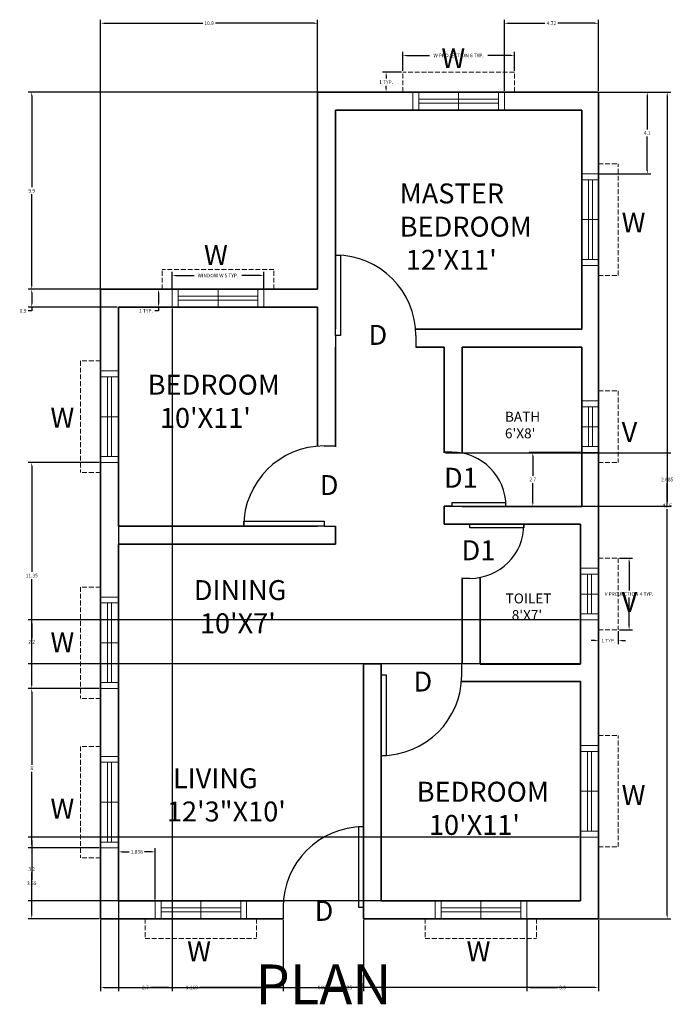
# Model space of a CAD drawing. Units: inches. Extents: x -193.8 to -127.9, y -122.4 to -72.3.
# Tile 1 of 2: x -193.8 to -161, y -122.4 to -73. Entities that reach past the tile are written whole.
import ezdxf

# ---------------------------------------------------------------- set-up
doc = ezdxf.new("R2010")
doc.units = ezdxf.units.IN
doc.header["$LTSCALE"] = 0.2
doc.header["$MEASUREMENT"] = 0
doc.linetypes.add('ACAD_ISO02W100', pattern=[15, 12, -3])
for name, color, linetype, lineweight in [('A-ANNO-DIMS', 2, 'Continuous', 18), ('A-ANNO-TEXT', 7, 'Continuous', 18), ('A-ANNO-TITL', 1, 'Continuous', 35), ('A-AREA-IDEN', 7, 'Continuous', 18), ('A-DOOR', 4, 'Continuous', 25), ('A-GLAZ', 4, 'Continuous', 18), ('A-GLAZ-OVHD', 8, 'ACAD_ISO02W100', 13), ('A-WALL', 7, 'Continuous', 35)]:
    doc.layers.add(name, color=color, linetype=linetype, lineweight=lineweight)
doc.styles.get("Standard").update_dxf_attribs({"font": 'arial.ttf'})
doc.dimstyles.get("Standard").update_dxf_attribs({"dimtxt": 0.18, "dimasz": 0.18, "dimexe": 0.18, "dimexo": 0.0625, "dimgap": 0.09, "dimtad": 0, "dimtih": 1, "dimtoh": 1, "dimdec": 1, "dimzin": 0, "dimdsep": 46, "dimlunit": 4, "dimtxsty": 'Standard', "dimcen": 0.09, "dimadec": 0, "dimazin": 0, "dimtfac": 1, "dimtdec": 1, "dimtofl": 0, "dimtmove": 0, "dimatfit": 3, "dimfxl": 1, "dimtolj": 1, "dimtzin": 0, "dimarcsym": 0})

# ---------------------------------------------------------------- blocks, each defined once
blk = doc.blocks.new('*U2')
for p, q in [((-700, 0), (-700, -100)), ((0, 0), (0, -100))]:
    blk.add_line(p, q)
blk.add_lwpolyline([(0, 0), (0, 700), (-43.75, 700), (-43.75, 0)], close=True)
blk.add_arc((0, 0), 700, 90, 180)
blk = doc.blocks.new('*U5')
for p, q in [((0, 0), (0, -100)), ((700, 0), (700, -100))]:
    blk.add_line(p, q)
blk.add_lwpolyline([(0, 0), (0, 700), (43.75, 700), (43.75, 0)], close=True)
blk.add_arc((0, 0), 700, 0, 90)
blk = doc.blocks.new('*U6')
for p, q in [((-700, 0), (-700, -100)), ((0, 0), (0, -100))]:
    blk.add_line(p, q)
blk.add_lwpolyline([(0, 0), (0, 700), (-43.75, 700), (-43.75, 0)], close=True)
blk.add_arc((0, 0), 700, 90, 180)
blk = doc.blocks.new('WIN-W-PLAN')
for p, q in [((0, 0.9), (0, 0)), ((0.3, 0.9), (0.3, 0)), ((0.3, 0.55), (4.3, 0.55)), ((2.3, 0.9), (2.3, 0)), ((4.3, 0.9), (4.3, 0)), ((4.6, 0.9), (4.6, 0)), ((0.3, 0.35), (4.3, 0.35))]:
    blk.add_line(p, q)
blk = doc.blocks.new('WIN-W-PROJECTION')
at = {"ltscale": 0.1}
for p, q in [((0.5, 1), (0, 1)), ((0, 1), (0, 0)), ((5.1, 1), (5.6, 1)), ((5.6, 1), (5.6, 0)), ((0, 0), (5.6, 0))]:
    blk.add_line(p, q, dxfattribs=at)
blk = doc.blocks.new('VENT-V-PROJECTION')
at = {"ltscale": 0.1}
for p, q in [((0, 3.1), (0, 3.6)), ((0, 3.6), (1, 3.6)), ((1, 3.6), (1, 0)), ((0, 0.5), (0, 0)), ((0, 0), (1, 0))]:
    blk.add_line(p, q, dxfattribs=at)
blk = doc.blocks.new('*D13')
at = {"layer": 'A-ANNO-DIMS', "color": 0, "lineweight": -2, "ltscale": 0.2, "transparency": 16777216}
for p, q in [((-186.171, -86.486), (-186.171, -85.678)), ((-185.991, -85.858), (-185.073, -85.858)), ((-181.751, -85.858), (-182.669, -85.858)), ((-181.571, -86.486), (-181.571, -85.678))]:
    blk.add_line(p, q, dxfattribs=at)
at = {"layer": 'A-ANNO-DIMS', "color": 0, "ltscale": 0.2, "transparency": 16777216}
for points in [[(-185.991, -85.828), (-185.991, -85.888), (-186.171, -85.858)], [(-181.751, -85.828), (-181.751, -85.888), (-181.571, -85.858)]]:
    blk.add_solid(points, dxfattribs=at)
at = {"layer": 'Defpoints', "color": 0, "ltscale": 0.2, "transparency": 16777216}
for p in [(-186.171, -85.858), (-186.171, -86.548), (-181.571, -86.548)]:
    blk.add_point(p, dxfattribs=at)
at = {"layer": 'A-ANNO-DIMS', "color": 0, "ltscale": 0.2, "transparency": 16777216, "insert": (-183.871, -85.858), "char_height": 0.18, "attachment_point": 5}
blk.add_mtext('\\A1;WINDOW W 5 TYP.', dxfattribs=at)
blk = doc.blocks.new('*D14')
at = {"layer": 'A-ANNO-DIMS', "color": 0, "lineweight": -2, "ltscale": 0.2, "transparency": 16777216}
for p, q in [((-186.234, -86.548), (-187.041, -86.548)), ((-186.861, -86.728), (-186.861, -87.268)), ((-186.234, -87.448), (-187.041, -87.448)), ((-186.861, -87.448), (-186.861, -87.628)), ((-186.861, -87.628), (-187.041, -87.628))]:
    blk.add_line(p, q, dxfattribs=at)
at = {"layer": 'A-ANNO-DIMS', "color": 0, "ltscale": 0.2, "transparency": 16777216}
for points in [[(-186.891, -86.728), (-186.831, -86.728), (-186.861, -86.548)], [(-186.891, -87.268), (-186.831, -87.268), (-186.861, -87.448)]]:
    blk.add_solid(points, dxfattribs=at)
at = {"layer": 'Defpoints', "color": 0, "ltscale": 0.2, "transparency": 16777216}
for p in [(-186.171, -86.548), (-186.861, -87.448), (-186.171, -87.448)]:
    blk.add_point(p, dxfattribs=at)
at = {"layer": 'A-ANNO-DIMS', "color": 0, "ltscale": 0.2, "transparency": 16777216, "insert": (-187.491, -87.628), "char_height": 0.18, "attachment_point": 5}
blk.add_mtext('\\A1;1 TYP.', dxfattribs=at)
blk = doc.blocks.new('*D15')
at = {"layer": 'A-ANNO-DIMS', "color": 0, "lineweight": -2, "ltscale": 0.2, "transparency": 16777216}
for p, q in [((-174.591, -75.586), (-174.591, -74.628)), ((-168.991, -75.586), (-168.991, -74.628)), ((-174.411, -74.808), (-173.252, -74.808)), ((-169.171, -74.808), (-170.331, -74.808))]:
    blk.add_line(p, q, dxfattribs=at)
at = {"layer": 'A-ANNO-DIMS', "color": 0, "ltscale": 0.2, "transparency": 16777216}
for points in [[(-174.411, -74.778), (-174.411, -74.838), (-174.591, -74.808)], [(-169.171, -74.778), (-169.171, -74.838), (-168.991, -74.808)]]:
    blk.add_solid(points, dxfattribs=at)
at = {"layer": 'Defpoints', "color": 0, "ltscale": 0.2, "transparency": 16777216}
for p in [(-174.591, -74.808), (-174.591, -75.648), (-168.991, -75.648)]:
    blk.add_point(p, dxfattribs=at)
at = {"layer": 'A-ANNO-DIMS', "color": 0, "ltscale": 0.2, "transparency": 16777216, "insert": (-171.791, -74.808), "char_height": 0.18, "attachment_point": 5}
blk.add_mtext('\\A1;W PROJECTION 6 TYP.', dxfattribs=at)
blk = doc.blocks.new('*D16')
at = {"layer": 'A-ANNO-DIMS', "color": 0, "lineweight": -2, "ltscale": 0.2, "transparency": 16777216}
for p, q in [((-174.654, -75.648), (-175.611, -75.648)), ((-175.431, -75.828), (-175.431, -75.968)), ((-175.431, -76.468), (-175.431, -76.329)), ((-174.654, -76.648), (-175.611, -76.648))]:
    blk.add_line(p, q, dxfattribs=at)
at = {"layer": 'A-ANNO-DIMS', "color": 0, "ltscale": 0.2, "transparency": 16777216}
for points in [[(-175.461, -75.828), (-175.401, -75.828), (-175.431, -75.648)], [(-175.461, -76.468), (-175.401, -76.468), (-175.431, -76.648)]]:
    blk.add_solid(points, dxfattribs=at)
at = {"layer": 'Defpoints', "color": 0, "ltscale": 0.2, "transparency": 16777216}
for p in [(-174.591, -75.648), (-175.431, -76.648), (-174.591, -76.648)]:
    blk.add_point(p, dxfattribs=at)
at = {"layer": 'A-ANNO-DIMS', "color": 0, "ltscale": 0.2, "transparency": 16777216, "insert": (-175.431, -76.148), "char_height": 0.18, "attachment_point": 5}
blk.add_mtext('\\A1;1 TYP.', dxfattribs=at)
blk = doc.blocks.new('*D17')
at = {"layer": 'A-ANNO-DIMS', "color": 0, "lineweight": -2, "ltscale": 0.2, "transparency": 16777216}
for p, q in [((-163.709, -100.048), (-163.051, -100.048)), ((-163.231, -100.228), (-163.231, -101.665)), ((-163.231, -103.468), (-163.231, -102.031)), ((-163.709, -103.648), (-163.051, -103.648))]:
    blk.add_line(p, q, dxfattribs=at)
at = {"layer": 'A-ANNO-DIMS', "color": 0, "ltscale": 0.2, "transparency": 16777216}
for points in [[(-163.261, -100.228), (-163.201, -100.228), (-163.231, -100.048)], [(-163.261, -103.468), (-163.201, -103.468), (-163.231, -103.648)]]:
    blk.add_solid(points, dxfattribs=at)
at = {"layer": 'Defpoints', "color": 0, "ltscale": 0.2, "transparency": 16777216}
for p in [(-163.771, -100.048), (-163.231, -100.048), (-163.771, -103.648)]:
    blk.add_point(p, dxfattribs=at)
at = {"layer": 'A-ANNO-DIMS', "color": 0, "ltscale": 0.2, "transparency": 16777216, "insert": (-163.231, -101.848), "char_height": 0.18, "attachment_point": 5}
blk.add_mtext('\\A1;V PROJECTION 4 TYP.', dxfattribs=at)
blk = doc.blocks.new('*D18')
at = {"layer": 'A-ANNO-DIMS', "color": 0, "lineweight": -2, "ltscale": 0.2, "transparency": 16777216}
for p, q in [((-164.771, -103.711), (-164.771, -104.368)), ((-163.771, -103.711), (-163.771, -104.368)), ((-164.951, -104.188), (-165.131, -104.188)), ((-163.591, -104.188), (-163.411, -104.188))]:
    blk.add_line(p, q, dxfattribs=at)
at = {"layer": 'A-ANNO-DIMS', "color": 0, "ltscale": 0.2, "transparency": 16777216}
for points in [[(-164.951, -104.158), (-164.951, -104.218), (-164.771, -104.188)], [(-163.591, -104.158), (-163.591, -104.218), (-163.771, -104.188)]]:
    blk.add_solid(points, dxfattribs=at)
at = {"layer": 'Defpoints', "color": 0, "ltscale": 0.2, "transparency": 16777216}
for p in [(-164.771, -103.648), (-163.771, -103.648), (-163.771, -104.188)]:
    blk.add_point(p, dxfattribs=at)
at = {"layer": 'A-ANNO-DIMS', "color": 0, "ltscale": 0.2, "transparency": 16777216, "insert": (-164.271, -104.188), "char_height": 0.18, "attachment_point": 5}
blk.add_mtext('\\A1;1 TYP.', dxfattribs=at)
blk = doc.blocks.new('*D25')
at = {"layer": 'A-ANNO-DIMS', "color": 0, "lineweight": -2, "ltscale": 0.2, "transparency": 16777216}
for p, q in [((-189.771, -118.211), (-189.771, -121.783)), ((-164.771, -118.211), (-164.771, -121.783)), ((-189.591, -121.603), (-177.492, -121.603)), ((-164.951, -121.603), (-177.05, -121.603))]:
    blk.add_line(p, q, dxfattribs=at)
at = {"layer": 'A-ANNO-DIMS', "color": 0, "ltscale": 0.2, "transparency": 16777216}
for points in [[(-189.591, -121.573), (-189.591, -121.633), (-189.771, -121.603)], [(-164.951, -121.573), (-164.951, -121.633), (-164.771, -121.603)]]:
    blk.add_solid(points, dxfattribs=at)
at = {"layer": 'Defpoints', "color": 0, "ltscale": 0.2, "transparency": 16777216}
for p in [(-189.771, -118.148), (-164.771, -118.148), (-164.771, -121.603)]:
    blk.add_point(p, dxfattribs=at)
at = {"layer": 'A-ANNO-DIMS', "color": 0, "ltscale": 0.2, "transparency": 16777216, "insert": (-177.271, -121.603), "char_height": 0.18, "attachment_point": 5}
blk.add_mtext('\\A1;25', dxfattribs=at)
blk = doc.blocks.new('*D26')
at = {"layer": 'A-ANNO-DIMS', "color": 0, "lineweight": -2, "ltscale": 0.2, "transparency": 16777216}
for p, q in [((-164.709, -76.648), (-161.136, -76.648)), ((-161.316, -76.828), (-161.316, -97.216)), ((-161.316, -117.968), (-161.316, -97.58)), ((-164.709, -118.148), (-161.136, -118.148))]:
    blk.add_line(p, q, dxfattribs=at)
at = {"layer": 'A-ANNO-DIMS', "color": 0, "ltscale": 0.2, "transparency": 16777216}
for points in [[(-161.346, -76.828), (-161.286, -76.828), (-161.316, -76.648)], [(-161.346, -117.968), (-161.286, -117.968), (-161.316, -118.148)]]:
    blk.add_solid(points, dxfattribs=at)
at = {"layer": 'Defpoints', "color": 0, "ltscale": 0.2, "transparency": 16777216}
for p in [(-164.771, -76.648), (-161.316, -76.648), (-164.771, -118.148)]:
    blk.add_point(p, dxfattribs=at)
at = {"layer": 'A-ANNO-DIMS', "color": 0, "ltscale": 0.2, "transparency": 16777216, "insert": (-161.316, -97.398), "char_height": 0.18, "attachment_point": 5}
blk.add_mtext('\\A1;41.5', dxfattribs=at)
blk = doc.blocks.new('*D27')
at = {"layer": 'A-ANNO-DIMS', "color": 0, "lineweight": -2, "ltscale": 0.2, "transparency": 16777216}
for p, q in [((-189.771, -86.486), (-189.771, -73.013)), ((-178.871, -86.486), (-178.871, -73.013)), ((-189.591, -73.193), (-184.637, -73.193)), ((-179.051, -73.193), (-184.006, -73.193))]:
    blk.add_line(p, q, dxfattribs=at)
at = {"layer": 'A-ANNO-DIMS', "color": 0, "ltscale": 0.2, "transparency": 16777216}
for points in [[(-189.591, -73.163), (-189.591, -73.223), (-189.771, -73.193)], [(-179.051, -73.163), (-179.051, -73.223), (-178.871, -73.193)]]:
    blk.add_solid(points, dxfattribs=at)
at = {"layer": 'Defpoints', "color": 0, "ltscale": 0.2, "transparency": 16777216}
for p in [(-178.871, -73.193), (-189.771, -86.548), (-178.871, -86.548)]:
    blk.add_point(p, dxfattribs=at)
at = {"layer": 'A-ANNO-DIMS', "color": 0, "ltscale": 0.2, "transparency": 16777216, "insert": (-184.321, -73.193), "char_height": 0.18, "attachment_point": 5}
blk.add_mtext('\\A1;10.9', dxfattribs=at)
blk = doc.blocks.new('*D28')
at = {"layer": 'A-ANNO-DIMS', "color": 0, "lineweight": -2, "ltscale": 0.2, "transparency": 16777216}
for p, q in [((-178.934, -76.648), (-193.406, -76.648)), ((-193.226, -76.828), (-193.226, -81.416)), ((-193.226, -86.368), (-193.226, -81.78)), ((-178.934, -86.548), (-193.406, -86.548))]:
    blk.add_line(p, q, dxfattribs=at)
at = {"layer": 'A-ANNO-DIMS', "color": 0, "ltscale": 0.2, "transparency": 16777216}
for points in [[(-193.256, -76.828), (-193.196, -76.828), (-193.226, -76.648)], [(-193.256, -86.368), (-193.196, -86.368), (-193.226, -86.548)]]:
    blk.add_solid(points, dxfattribs=at)
at = {"layer": 'Defpoints', "color": 0, "ltscale": 0.2, "transparency": 16777216}
for p in [(-193.226, -76.648), (-178.871, -76.648), (-178.871, -86.548)]:
    blk.add_point(p, dxfattribs=at)
at = {"layer": 'A-ANNO-DIMS', "color": 0, "ltscale": 0.2, "transparency": 16777216, "insert": (-193.226, -81.598), "char_height": 0.18, "attachment_point": 5}
blk.add_mtext('\\A1;9.9', dxfattribs=at)
blk = doc.blocks.new('*D29')
at = {"layer": 'A-ANNO-DIMS', "color": 0, "lineweight": -2, "ltscale": 0.2, "transparency": 16777216}
for p, q in [((-189.771, -118.211), (-189.771, -121.783)), ((-180.602, -118.211), (-180.602, -121.783)), ((-189.591, -121.603), (-185.581, -121.603)), ((-180.782, -121.603), (-184.793, -121.603))]:
    blk.add_line(p, q, dxfattribs=at)
at = {"layer": 'A-ANNO-DIMS', "color": 0, "ltscale": 0.2, "transparency": 16777216}
for points in [[(-189.591, -121.573), (-189.591, -121.633), (-189.771, -121.603)], [(-180.782, -121.573), (-180.782, -121.633), (-180.602, -121.603)]]:
    blk.add_solid(points, dxfattribs=at)
at = {"layer": 'Defpoints', "color": 0, "ltscale": 0.2, "transparency": 16777216}
for p in [(-189.771, -118.148), (-180.602, -118.148), (-180.602, -121.603)]:
    blk.add_point(p, dxfattribs=at)
at = {"layer": 'A-ANNO-DIMS', "color": 0, "ltscale": 0.2, "transparency": 16777216, "insert": (-185.187, -121.603), "char_height": 0.18, "attachment_point": 5}
blk.add_mtext('\\A1;9.169', dxfattribs=at)
blk = doc.blocks.new('*D30')
at = {"layer": 'A-ANNO-DIMS', "color": 0, "lineweight": -2, "ltscale": 0.2, "transparency": 16777216}
for p, q in [((-180.602, -118.211), (-180.602, -121.783)), ((-176.571, -118.211), (-176.571, -121.783)), ((-180.422, -121.603), (-178.967, -121.603)), ((-176.751, -121.603), (-178.207, -121.603))]:
    blk.add_line(p, q, dxfattribs=at)
at = {"layer": 'A-ANNO-DIMS', "color": 0, "ltscale": 0.2, "transparency": 16777216}
for points in [[(-180.422, -121.573), (-180.422, -121.633), (-180.602, -121.603)], [(-176.751, -121.573), (-176.751, -121.633), (-176.571, -121.603)]]:
    blk.add_solid(points, dxfattribs=at)
at = {"layer": 'Defpoints', "color": 0, "ltscale": 0.2, "transparency": 16777216}
for p in [(-180.602, -118.148), (-176.571, -118.148), (-176.571, -121.603)]:
    blk.add_point(p, dxfattribs=at)
at = {"layer": 'A-ANNO-DIMS', "color": 0, "ltscale": 0.2, "transparency": 16777216, "insert": (-178.587, -121.603), "char_height": 0.18, "attachment_point": 5}
blk.add_mtext('\\A1;4.031', dxfattribs=at)
blk = doc.blocks.new('*D31')
at = {"layer": 'A-ANNO-DIMS', "color": 0, "lineweight": -2, "ltscale": 0.2, "transparency": 16777216}
for p, q in [((-172.449, -94.756), (-161.136, -94.756)), ((-161.316, -94.936), (-161.316, -95.917)), ((-161.316, -97.261), (-161.316, -96.281)), ((-172.449, -97.441), (-161.136, -97.441))]:
    blk.add_line(p, q, dxfattribs=at)
at = {"layer": 'A-ANNO-DIMS', "color": 0, "ltscale": 0.2, "transparency": 16777216}
for points in [[(-161.346, -94.936), (-161.286, -94.936), (-161.316, -94.756)], [(-161.346, -97.261), (-161.286, -97.261), (-161.316, -97.441)]]:
    blk.add_solid(points, dxfattribs=at)
at = {"layer": 'Defpoints', "color": 0, "ltscale": 0.2, "transparency": 16777216}
for p in [(-172.511, -94.756), (-172.511, -97.441), (-161.316, -97.441)]:
    blk.add_point(p, dxfattribs=at)
at = {"layer": 'A-ANNO-DIMS', "color": 0, "ltscale": 0.2, "transparency": 16777216, "insert": (-161.316, -96.099), "char_height": 0.18, "attachment_point": 5}
blk.add_mtext('\\A1;2.685', dxfattribs=at)
blk = doc.blocks.new('*D32')
at = {"layer": 'A-ANNO-DIMS', "color": 0, "lineweight": -2, "ltscale": 0.2, "transparency": 16777216}
for p, q in [((-189.834, -86.548), (-193.406, -86.548)), ((-193.226, -86.728), (-193.226, -87.268)), ((-188.934, -87.448), (-193.406, -87.448)), ((-193.226, -87.448), (-193.226, -87.628)), ((-193.226, -87.628), (-193.406, -87.628))]:
    blk.add_line(p, q, dxfattribs=at)
at = {"layer": 'A-ANNO-DIMS', "color": 0, "ltscale": 0.2, "transparency": 16777216}
for points in [[(-193.256, -86.728), (-193.196, -86.728), (-193.226, -86.548)], [(-193.256, -87.268), (-193.196, -87.268), (-193.226, -87.448)]]:
    blk.add_solid(points, dxfattribs=at)
at = {"layer": 'Defpoints', "color": 0, "ltscale": 0.2, "transparency": 16777216}
for p in [(-189.771, -86.548), (-193.226, -87.448), (-188.871, -87.448)]:
    blk.add_point(p, dxfattribs=at)
at = {"layer": 'A-ANNO-DIMS', "color": 0, "ltscale": 0.2, "transparency": 16777216, "insert": (-193.66, -87.628), "char_height": 0.18, "attachment_point": 5}
blk.add_mtext('\\A1;0.9', dxfattribs=at)
blk = doc.blocks.new('*D33')
at = {"layer": 'A-ANNO-DIMS', "color": 0, "lineweight": -2, "ltscale": 0.2, "transparency": 16777216}
for p, q in [((-189.834, -114.598), (-193.406, -114.598)), ((-193.226, -114.778), (-193.226, -116.191)), ((-193.226, -117.968), (-193.226, -116.555)), ((-189.834, -118.148), (-193.406, -118.148))]:
    blk.add_line(p, q, dxfattribs=at)
at = {"layer": 'A-ANNO-DIMS', "color": 0, "ltscale": 0.2, "transparency": 16777216}
for points in [[(-193.256, -114.778), (-193.196, -114.778), (-193.226, -114.598)], [(-193.256, -117.968), (-193.196, -117.968), (-193.226, -118.148)]]:
    blk.add_solid(points, dxfattribs=at)
at = {"layer": 'Defpoints', "color": 0, "ltscale": 0.2, "transparency": 16777216}
for p in [(-193.226, -114.598), (-189.771, -114.598), (-189.771, -118.148)]:
    blk.add_point(p, dxfattribs=at)
at = {"layer": 'A-ANNO-DIMS', "color": 0, "ltscale": 0.2, "transparency": 16777216, "insert": (-193.226, -116.373), "char_height": 0.18, "attachment_point": 5}
blk.add_mtext('\\A1;3.55', dxfattribs=at)
blk = doc.blocks.new('*D34')
at = {"layer": 'A-ANNO-DIMS', "color": 0, "lineweight": -2, "ltscale": 0.2, "transparency": 16777216}
for p, q in [((-189.834, -106.598), (-193.406, -106.598)), ((-193.226, -106.778), (-193.226, -110.416)), ((-193.226, -114.418), (-193.226, -110.78)), ((-189.834, -114.598), (-193.406, -114.598))]:
    blk.add_line(p, q, dxfattribs=at)
at = {"layer": 'A-ANNO-DIMS', "color": 0, "ltscale": 0.2, "transparency": 16777216}
for points in [[(-193.256, -106.778), (-193.196, -106.778), (-193.226, -106.598)], [(-193.256, -114.418), (-193.196, -114.418), (-193.226, -114.598)]]:
    blk.add_solid(points, dxfattribs=at)
at = {"layer": 'Defpoints', "color": 0, "ltscale": 0.2, "transparency": 16777216}
for p in [(-193.226, -106.598), (-189.771, -106.598), (-189.771, -114.598)]:
    blk.add_point(p, dxfattribs=at)
at = {"layer": 'A-ANNO-DIMS', "color": 0, "ltscale": 0.2, "transparency": 16777216, "insert": (-193.226, -110.598), "char_height": 0.18, "attachment_point": 5}
blk.add_mtext('\\A1;8', dxfattribs=at)
blk = doc.blocks.new('*D35')
at = {"layer": 'A-ANNO-DIMS', "color": 0, "lineweight": -2, "ltscale": 0.2, "transparency": 16777216}
for p, q in [((-189.834, -95.248), (-193.406, -95.248)), ((-193.226, -95.428), (-193.226, -100.741)), ((-193.226, -106.418), (-193.226, -101.105)), ((-189.834, -106.598), (-193.406, -106.598))]:
    blk.add_line(p, q, dxfattribs=at)
at = {"layer": 'A-ANNO-DIMS', "color": 0, "ltscale": 0.2, "transparency": 16777216}
for points in [[(-193.256, -95.428), (-193.196, -95.428), (-193.226, -95.248)], [(-193.256, -106.418), (-193.196, -106.418), (-193.226, -106.598)]]:
    blk.add_solid(points, dxfattribs=at)
at = {"layer": 'Defpoints', "color": 0, "ltscale": 0.2, "transparency": 16777216}
for p in [(-193.226, -95.248), (-189.771, -95.248), (-189.771, -106.598)]:
    blk.add_point(p, dxfattribs=at)
at = {"layer": 'A-ANNO-DIMS', "color": 0, "ltscale": 0.2, "transparency": 16777216, "insert": (-193.226, -100.923), "char_height": 0.18, "attachment_point": 5}
blk.add_mtext('\\A1;11.35', dxfattribs=at)
blk = doc.blocks.new('*D36')
at = {"layer": 'A-ANNO-DIMS', "color": 0, "lineweight": -2, "ltscale": 0.2, "transparency": 16777216}
for p, q in [((-168.371, -118.211), (-168.371, -121.783)), ((-164.771, -118.211), (-164.771, -121.783)), ((-168.191, -121.603), (-166.825, -121.603)), ((-164.951, -121.603), (-166.318, -121.603))]:
    blk.add_line(p, q, dxfattribs=at)
at = {"layer": 'A-ANNO-DIMS', "color": 0, "ltscale": 0.2, "transparency": 16777216}
for points in [[(-168.191, -121.573), (-168.191, -121.633), (-168.371, -121.603)], [(-164.951, -121.573), (-164.951, -121.633), (-164.771, -121.603)]]:
    blk.add_solid(points, dxfattribs=at)
at = {"layer": 'Defpoints', "color": 0, "ltscale": 0.2, "transparency": 16777216}
for p in [(-168.371, -118.148), (-164.771, -118.148), (-168.371, -121.603)]:
    blk.add_point(p, dxfattribs=at)
at = {"layer": 'A-ANNO-DIMS', "color": 0, "ltscale": 0.2, "transparency": 16777216, "insert": (-166.571, -121.603), "char_height": 0.18, "attachment_point": 5}
blk.add_mtext('\\A1;3.6', dxfattribs=at)
blk = doc.blocks.new('*D37')
at = {"layer": 'A-ANNO-DIMS', "color": 0, "lineweight": -2, "ltscale": 0.2, "transparency": 16777216}
for p, q in [((-188.871, -87.511), (-188.871, -121.783)), ((-186.171, -87.511), (-186.171, -121.783)), ((-188.691, -121.603), (-187.777, -121.603)), ((-186.351, -121.603), (-187.266, -121.603))]:
    blk.add_line(p, q, dxfattribs=at)
at = {"layer": 'A-ANNO-DIMS', "color": 0, "ltscale": 0.2, "transparency": 16777216}
for points in [[(-188.691, -121.573), (-188.691, -121.633), (-188.871, -121.603)], [(-186.351, -121.573), (-186.351, -121.633), (-186.171, -121.603)]]:
    blk.add_solid(points, dxfattribs=at)
at = {"layer": 'Defpoints', "color": 0, "ltscale": 0.2, "transparency": 16777216}
for p in [(-188.871, -87.448), (-186.171, -87.448), (-186.171, -121.603)]:
    blk.add_point(p, dxfattribs=at)
at = {"layer": 'A-ANNO-DIMS', "color": 0, "ltscale": 0.2, "transparency": 16777216, "insert": (-187.521, -121.603), "char_height": 0.18, "attachment_point": 5}
blk.add_mtext('\\A1;2.7', dxfattribs=at)
blk = doc.blocks.new('*D38')
at = {"layer": 'A-ANNO-DIMS', "color": 0, "lineweight": -2, "ltscale": 0.2, "transparency": 16777216}
for p, q in [((-169.491, -76.586), (-169.491, -73.013)), ((-164.771, -76.586), (-164.771, -73.013)), ((-169.311, -73.193), (-167.458, -73.193)), ((-164.951, -73.193), (-166.805, -73.193))]:
    blk.add_line(p, q, dxfattribs=at)
at = {"layer": 'A-ANNO-DIMS', "color": 0, "ltscale": 0.2, "transparency": 16777216}
for points in [[(-169.311, -73.163), (-169.311, -73.223), (-169.491, -73.193)], [(-164.951, -73.163), (-164.951, -73.223), (-164.771, -73.193)]]:
    blk.add_solid(points, dxfattribs=at)
at = {"layer": 'Defpoints', "color": 0, "ltscale": 0.2, "transparency": 16777216}
for p in [(-169.491, -73.193), (-169.491, -76.648), (-164.771, -76.648)]:
    blk.add_point(p, dxfattribs=at)
at = {"layer": 'A-ANNO-DIMS', "color": 0, "ltscale": 0.2, "transparency": 16777216, "insert": (-167.131, -73.193), "char_height": 0.18, "attachment_point": 5}
blk.add_mtext('\\A1;4.72', dxfattribs=at)
blk = doc.blocks.new('*D39')
at = {"layer": 'A-ANNO-DIMS', "color": 0, "lineweight": -2, "ltscale": 0.2, "transparency": 16777216}
for p, q in [((-164.709, -76.648), (-162.136, -76.648)), ((-162.316, -76.828), (-162.316, -78.518)), ((-162.316, -80.568), (-162.316, -78.879)), ((-164.709, -80.748), (-162.136, -80.748))]:
    blk.add_line(p, q, dxfattribs=at)
at = {"layer": 'A-ANNO-DIMS', "color": 0, "ltscale": 0.2, "transparency": 16777216}
for points in [[(-162.346, -76.828), (-162.286, -76.828), (-162.316, -76.648)], [(-162.346, -80.568), (-162.286, -80.568), (-162.316, -80.748)]]:
    blk.add_solid(points, dxfattribs=at)
at = {"layer": 'Defpoints', "color": 0, "ltscale": 0.2, "transparency": 16777216}
for p in [(-164.771, -76.648), (-164.771, -80.748), (-162.316, -80.748)]:
    blk.add_point(p, dxfattribs=at)
at = {"layer": 'A-ANNO-DIMS', "color": 0, "ltscale": 0.2, "transparency": 16777216, "insert": (-162.316, -78.698), "char_height": 0.18, "attachment_point": 5}
blk.add_mtext('\\A1;4.1', dxfattribs=at)
blk = doc.blocks.new('*D40')
at = {"layer": 'A-ANNO-DIMS', "color": 0, "lineweight": -2, "ltscale": 0.2, "transparency": 16777216}
for p, q in [((-165.734, -114.048), (-193.406, -114.048)), ((-193.226, -114.228), (-193.226, -115.466)), ((-193.226, -117.068), (-193.226, -115.83)), ((-165.734, -117.248), (-193.406, -117.248))]:
    blk.add_line(p, q, dxfattribs=at)
at = {"layer": 'A-ANNO-DIMS', "color": 0, "ltscale": 0.2, "transparency": 16777216}
for points in [[(-193.256, -114.228), (-193.196, -114.228), (-193.226, -114.048)], [(-193.256, -117.068), (-193.196, -117.068), (-193.226, -117.248)]]:
    blk.add_solid(points, dxfattribs=at)
at = {"layer": 'Defpoints', "color": 0, "ltscale": 0.2, "transparency": 16777216}
for p in [(-193.226, -114.048), (-165.671, -114.048), (-165.671, -117.248)]:
    blk.add_point(p, dxfattribs=at)
at = {"layer": 'A-ANNO-DIMS', "color": 0, "ltscale": 0.2, "transparency": 16777216, "insert": (-193.226, -115.648), "char_height": 0.18, "attachment_point": 5}
blk.add_mtext('\\A1;3.2', dxfattribs=at)
blk = doc.blocks.new('*D41')
at = {"layer": 'A-ANNO-DIMS', "color": 0, "lineweight": -2, "ltscale": 0.2, "transparency": 16777216}
for p, q in [((-165.674, -94.748), (-168.246, -94.748)), ((-168.066, -94.928), (-168.066, -95.918)), ((-168.066, -97.268), (-168.066, -96.279)), ((-165.674, -97.448), (-168.246, -97.448))]:
    blk.add_line(p, q, dxfattribs=at)
at = {"layer": 'A-ANNO-DIMS', "color": 0, "ltscale": 0.2, "transparency": 16777216}
for points in [[(-168.096, -94.928), (-168.036, -94.928), (-168.066, -94.748)], [(-168.096, -97.268), (-168.036, -97.268), (-168.066, -97.448)]]:
    blk.add_solid(points, dxfattribs=at)
at = {"layer": 'Defpoints', "color": 0, "ltscale": 0.2, "transparency": 16777216}
for p in [(-168.066, -94.748), (-165.611, -94.748), (-165.611, -97.448)]:
    blk.add_point(p, dxfattribs=at)
at = {"layer": 'A-ANNO-DIMS', "color": 0, "ltscale": 0.2, "transparency": 16777216, "insert": (-168.066, -96.098), "char_height": 0.18, "attachment_point": 5}
blk.add_mtext('\\A1;2.7', dxfattribs=at)
blk = doc.blocks.new('*D42')
at = {"layer": 'A-ANNO-DIMS', "color": 0, "lineweight": -2, "ltscale": 0.2, "transparency": 16777216}
for p, q in [((-165.734, -103.148), (-193.406, -103.148)), ((-193.226, -103.328), (-193.226, -104.068)), ((-193.226, -105.168), (-193.226, -104.429)), ((-165.734, -105.348), (-193.406, -105.348))]:
    blk.add_line(p, q, dxfattribs=at)
at = {"layer": 'A-ANNO-DIMS', "color": 0, "ltscale": 0.2, "transparency": 16777216}
for points in [[(-193.256, -103.328), (-193.196, -103.328), (-193.226, -103.148)], [(-193.256, -105.168), (-193.196, -105.168), (-193.226, -105.348)]]:
    blk.add_solid(points, dxfattribs=at)
at = {"layer": 'Defpoints', "color": 0, "ltscale": 0.2, "transparency": 16777216}
for p in [(-193.226, -103.148), (-165.671, -103.148), (-165.671, -105.348)]:
    blk.add_point(p, dxfattribs=at)
at = {"layer": 'A-ANNO-DIMS', "color": 0, "ltscale": 0.2, "transparency": 16777216, "insert": (-193.226, -104.248), "char_height": 0.18, "attachment_point": 5}
blk.add_mtext('\\A1;2.2', dxfattribs=at)
blk = doc.blocks.new('*D43')
at = {"layer": 'A-ANNO-DIMS', "color": 0, "lineweight": -2, "ltscale": 0.2, "transparency": 16777216}
for p, q in [((-188.871, -117.186), (-188.871, -114.613)), ((-187.033, -117.186), (-187.033, -114.613)), ((-188.691, -114.793), (-188.338, -114.793)), ((-187.213, -114.793), (-187.567, -114.793))]:
    blk.add_line(p, q, dxfattribs=at)
at = {"layer": 'A-ANNO-DIMS', "color": 0, "ltscale": 0.2, "transparency": 16777216}
for points in [[(-188.691, -114.763), (-188.691, -114.823), (-188.871, -114.793)], [(-187.213, -114.763), (-187.213, -114.823), (-187.033, -114.793)]]:
    blk.add_solid(points, dxfattribs=at)
at = {"layer": 'Defpoints', "color": 0, "ltscale": 0.2, "transparency": 16777216}
for p in [(-187.033, -114.793), (-188.871, -117.248), (-187.033, -117.248)]:
    blk.add_point(p, dxfattribs=at)
at = {"layer": 'A-ANNO-DIMS', "color": 0, "ltscale": 0.2, "transparency": 16777216, "insert": (-187.952, -114.793), "char_height": 0.18, "attachment_point": 5}
blk.add_mtext('\\A1;1.838', dxfattribs=at)

msp = doc.modelspace()

# ---------------------------------------------------------------- linework, layer by layer
at = {"layer": 'A-GLAZ'}
for p, q in [((-165.6113, -80.7483), (-164.7714, -80.7483)), ((-165.6113, -81.0483), (-164.7714, -81.0483)), ((-165.2613, -81.0483), (-165.2613, -85.0483)), ((-165.0613, -81.0483), (-165.0613, -85.0483)), ((-165.6113, -83.0483), (-164.7714, -83.0483)), ((-165.6113, -85.0483), (-164.7714, -85.0483)), ((-165.6113, -85.3483), (-164.7714, -85.3483)), ((-165.6113, -92.1483), (-164.7714, -92.1483)), ((-165.6113, -92.4483), (-164.7714, -92.4483)), ((-165.2613, -92.4483), (-165.2613, -94.4483)), ((-165.0613, -92.4483), (-165.0613, -94.4483)), ((-165.6113, -93.4483), (-164.7714, -93.4483)), ((-165.6113, -94.4483), (-164.7714, -94.4483)), ((-165.6113, -94.7483), (-164.7714, -94.7483)), ((-165.6714, -100.5483), (-164.7714, -100.5483)), ((-165.6714, -100.8483), (-164.7714, -100.8483)), ((-165.3214, -100.8483), (-165.3214, -102.8483)), ((-165.1214, -100.8483), (-165.1214, -102.8483)), ((-165.6714, -101.8483), (-164.7714, -101.8483)), ((-165.6714, -102.8483), (-164.7714, -102.8483)), ((-165.6714, -103.1483), (-164.7714, -103.1483))]:
    msp.add_line(p, q, dxfattribs=at)
at = {"layer": 'A-GLAZ-OVHD', "ltscale": 0.1}
msp.add_line((-182.4334, -117.2483), (-181.9334, -117.2483), dxfattribs=at)
at = {"layer": 'A-WALL'}
for p, q in [((-178.8714, -76.6483), (-178.8714, -86.5483)), ((-164.7714, -76.6483), (-178.8714, -76.6483)), ((-164.7714, -105.3483), (-164.7714, -76.6483)), ((-177.9714, -77.5483), (-177.9714, -88.5483)), ((-165.6113, -77.5483), (-177.9714, -77.5483)), ((-165.6113, -88.5483), (-165.6113, -77.5483)), ((-189.7714, -99.3483), (-189.7714, -86.5483)), ((-189.7714, -86.5483), (-178.8714, -86.5483)), ((-188.8714, -87.4483), (-178.8714, -87.4483)), ((-188.8714, -98.4483), (-188.8714, -87.4483)), ((-178.8714, -87.4483), (-178.8714, -94.4269)), ((-178.8714, -87.4483), (-178.8714, -94.4269)), ((-173.9492, -88.5483), (-165.6113, -88.5483)), ((-165.6113, -88.5483), (-171.6113, -88.5483)), ((-177.9714, -89.4483), (-177.9714, -94.4553)), ((-173.9362, -89.4483), (-172.5113, -89.4483)), ((-172.5113, -89.4483), (-172.5113, -94.7565)), ((-165.6113, -89.4483), (-171.6113, -89.4483)), ((-171.6113, -89.4483), (-165.6113, -89.4483)), ((-171.6113, -89.4483), (-171.6113, -94.7775)), ((-165.6113, -97.4483), (-165.6113, -89.4483)), ((-172.5113, -97.4413), (-172.5113, -98.3483)), ((-171.6113, -97.4413), (-171.6113, -97.4483)), ((-165.6113, -97.4483), (-171.6113, -97.4483)), ((-165.6714, -98.3483), (-172.5113, -98.3483)), ((-171.6113, -98.3483), (-172.5113, -98.3483)), ((-165.6714, -105.3483), (-165.6714, -98.3483)), ((-189.7714, -98.4483), (-189.7714, -118.1483)), ((-178.8714, -98.4483), (-188.8714, -98.4483)), ((-177.9714, -98.4483), (-177.9714, -99.3483)), ((-177.9714, -99.3483), (-188.8714, -99.3483)), ((-188.8714, -99.3483), (-188.8714, -117.2483)), ((-171.6113, -101.0331), (-171.6113, -105.3483)), ((-170.7113, -101.012), (-170.7113, -105.3483)), ((-176.5714, -117.2483), (-176.5714, -105.3483)), ((-175.6714, -105.3483), (-176.5714, -105.3483)), ((-175.6714, -105.3483), (-175.6714, -117.2483)), ((-171.6362, -105.3764), (-171.6113, -105.3764)), ((-170.7113, -105.3764), (-165.6714, -105.3764)), ((-164.7714, -118.1483), (-164.7714, -105.3483)), ((-165.6714, -106.2483), (-171.6492, -106.2483)), ((-165.6714, -117.2483), (-165.6714, -106.2483)), ((-175.6714, -117.2483), (-175.6714, -107.2483)), ((-188.8714, -117.2483), (-180.5955, -117.2483)), ((-176.5714, -117.2483), (-176.5714, -118.1483)), ((-175.6714, -117.2483), (-165.6714, -117.2483)), ((-189.7714, -118.1483), (-180.6024, -118.1483)), ((-176.5714, -118.1483), (-164.7714, -118.1483))]:
    msp.add_line(p, q, dxfattribs=at)

# ---------------------------------------------------------------- block references
at = {"layer": 'A-DOOR', "xscale": 0.0057645088651403, "yscale": 0.0057645088651403, "zscale": 0.0057645088651403}
for name, p in [('*U5', (-177.9714, -88.8718)), ('*U2', (-176.5672, -117.5718))]:
    msp.add_blockref(name, p, dxfattribs=at)
at = {"layer": 'A-DOOR'}
for name, p, xscale, yscale, zscale, rotation in [('*U5', (-178.5478, -98.4491), 0.0057645088651403, 0.0057645088651403, 0.0057645088651403, 90), ('*U6', (-172.1238, -97.4413), 0.0038751449514543, 0.0038751449514543, 0.0038751449514543, 270), ('*U5', (-171.2238, -98.3483), 0.0038751449514543, 0.0038751449514543, 0.0038751449514543, 270), ('*U2', (-175.6714, -105.9247), 0.0057645088651403, 0.0057645088651403, 0.0057645088651403, 180)]:
    msp.add_blockref(name, p, dxfattribs=dict(at, xscale=xscale, yscale=yscale, zscale=zscale, rotation=rotation))
at = {"layer": 'A-GLAZ'}
for p, rotation in [((-169.4913, -76.6483), 180), ((-181.5714, -86.5483), 180), ((-188.8714, -95.2483), 90.00000000000003), ((-189.7714, -101.9983), 270.0000000000013), ((-165.6714, -109.4483), 269.9999999999996), ((-189.7714, -109.9983), 270.0000000000008), ((-182.4334, -117.2483), 180)]:
    msp.add_blockref('WIN-W-PLAN', p, dxfattribs=dict(at, rotation=rotation))
msp.add_blockref('WIN-W-PLAN', (-172.9714, -118.1483), dxfattribs=at)
at = {"layer": 'A-GLAZ-OVHD'}
for p, rotation in [((-168.9913, -75.6483), 180), ((-163.7714, -85.8483), 90.00000000000044), ((-181.0714, -85.5483), 180), ((-190.7714, -90.1483), 270.0000000000015), ((-190.7714, -101.4983), 270.0000000000012), ((-163.7714, -114.5483), 89.99999999999876), ((-190.7714, -109.4983), 270.0000000000017)]:
    msp.add_blockref('WIN-W-PROJECTION', p, dxfattribs=dict(at, rotation=rotation))
for name, p in [('VENT-V-PROJECTION', (-164.7714, -95.2483)), ('VENT-V-PROJECTION', (-164.7714, -103.6483)), ('WIN-W-PROJECTION', (-187.5334, -119.1483)), ('WIN-W-PROJECTION', (-173.4714, -119.1483))]:
    msp.add_blockref(name, p, dxfattribs=at)

# ---------------------------------------------------------------- texts
at = {"layer": 'A-ANNO-TEXT'}
for s, p in [('W', (-172.6574, -75.4453)), ('W', (-163.6049, -83.6935)), ('W', (-184.5769, -85.3254)), ('D', (-176.3139, -89.3385)), ('W', (-192.2872, -93.4984)), ('V', (-163.6049, -94.2107)), ('D', (-178.7616, -96.8775)), ('D1', (-172.5277, -96.5098)), ('D1', (-171.6439, -100.1523)), ('V', (-163.6049, -102.7455)), ('W', (-192.2872, -104.7676)), ('D', (-174.0549, -106.743)), ('W', (-163.6049, -112.4407)), ('W', (-192.2872, -113.1263)), ('D', (-179.0211, -118.2563)), ('W', (-185.4237, -120.2827)), ('W', (-171.3904, -120.2827))]:
    msp.add_text(s, height=1, dxfattribs=at).set_placement(p)
at = {"layer": 'A-ANNO-TITL', "ltscale": 0.2}
msp.add_text('PLAN', height=2, dxfattribs=at).set_placement((-181.9971, -122.4469))
at = {"layer": 'A-AREA-IDEN', "attachment_point": 1}
for s, insert, char_height in [("MASTER BEDROOM\\P 12'X11'", (-174.7481, -81.2369), 1), ("BEDROOM\\P  10'X11'", (-187.4018, -90.8385), 1), ("BATH\\P6'X8'", (-169.4632, -92.6973), 0.5), ("DINING\\P 10'X7'", (-185.0881, -101.1507), 1), ("TOILET\\P  8'X7'", (-169.427, -101.8214), 0.5), (' LIVING   12\'3"X10\'', (-186.4393, -110.5988), 1), ("BEDROOM\\P  10'X11'", (-173.8927, -111.2737), 1)]:
    msp.add_mtext_dynamic_manual_height_columns(s, width=5.597724, gutter_width=5.1307, heights=[0], dxfattribs=dict(at, insert=insert, char_height=char_height))

# ---------------------------------------------------------------- dimensions: what is measured, and where the dimension line sits
at = {"layer": 'A-ANNO-DIMS', "ltscale": 0.2}
for base, p1, p2, override, picture, middle in [((-178.8714, -73.1933), (-189.7714, -86.5483), (-178.8714, -86.5483), {"dimdec": 1, "dimlfac": 1, "dimrnd": 0, "dimzin": 0, "dimdsep": 46, "dimlunit": 2}, '*D27', (-184.3214, -73.1933)), ((-169.4913, -73.1933), (-164.7714, -76.6483), (-169.4913, -76.6483), {"dimdec": 2, "dimlfac": 1, "dimrnd": 0, "dimzin": 0, "dimdsep": 46, "dimlunit": 2}, '*D38', (-167.1314, -73.1933)), ((-186.1714, -121.6033), (-188.8714, -87.4483), (-186.1714, -87.4483), {"dimdec": 1, "dimlfac": 1, "dimrnd": 0, "dimzin": 0, "dimdsep": 46, "dimlunit": 2}, '*D37', (-187.5214, -121.6033)), ((-187.0334, -114.7933), (-188.8714, -117.2483), (-187.0334, -117.2483), {"dimdec": 3, "dimlfac": 1, "dimrnd": 0, "dimzin": 0, "dimdsep": 46, "dimlunit": 2}, '*D43', (-187.9524, -114.7933)), ((-164.7714, -121.6033), (-189.7714, -118.1483), (-164.7714, -118.1483), {"dimdec": 0, "dimlfac": 1, "dimrnd": 0, "dimzin": 0, "dimdsep": 46, "dimlunit": 2}, '*D25', (-177.2714, -121.6033)), ((-180.6024, -121.6033), (-189.7714, -118.1483), (-180.6024, -118.1483), {"dimdec": 3, "dimlfac": 1, "dimrnd": 0, "dimzin": 0, "dimdsep": 46, "dimlunit": 2}, '*D29', (-185.1869, -121.6033)), ((-176.5714, -121.6033), (-180.6024, -118.1483), (-176.5714, -118.1483), {"dimdec": 3, "dimlfac": 1, "dimrnd": 0, "dimzin": 0, "dimdsep": 46, "dimlunit": 2}, '*D30', (-178.5869, -121.6033)), ((-168.3714, -121.6033), (-164.7714, -118.1483), (-168.3714, -118.1483), {"dimdec": 1, "dimlfac": 1, "dimrnd": 0, "dimzin": 0, "dimdsep": 46, "dimlunit": 2}, '*D36', (-166.5714, -121.6033))]:
    dim = msp.add_linear_dim(base=base, p1=p1, p2=p2, dimstyle='Standard', override=override, dxfattribs=at)
    dim.commit()
    dim.dimension.update_dxf_attribs({"geometry": picture, "text_midpoint": middle})
for base, p1, p2, angle, text, picture, middle in [((-174.5913, -74.8083), (-168.9913, -75.6483), (-174.5913, -75.6483), 180, 'W PROJECTION <> TYP.', '*D15', (-171.7913, -74.8083)), ((-175.4313, -76.6483), (-174.5913, -75.6483), (-174.5913, -76.6483), 270, '<> TYP.', '*D16', (-175.4313, -76.1483)), ((-186.1714, -85.8583), (-181.5714, -86.5483), (-186.1714, -86.5483), 180, 'WINDOW W <> TYP.', '*D13', (-183.8714, -85.8583)), ((-186.8614, -87.4483), (-186.1714, -86.5483), (-186.1714, -87.4483), 270, '<> TYP.', '*D14', (-187.491, -87.6283)), ((-163.2314, -100.0483), (-163.7714, -103.6483), (-163.7714, -100.0483), 90, 'V PROJECTION <> TYP.', '*D17', (-163.2314, -101.8483))]:
    dim = msp.add_linear_dim(base=base, p1=p1, p2=p2, angle=angle, text=text, dimstyle='Standard', override={"dimdec": 0, "dimlfac": 1, "dimrnd": 0, "dimzin": 0, "dimdsep": 46, "dimlunit": 2}, dxfattribs=at)
    dim.commit()
    dim.dimension.update_dxf_attribs({"geometry": picture, "text_midpoint": middle})
for base, p1, p2, angle, override, picture, middle in [((-193.2264, -76.6483), (-178.8714, -86.5483), (-178.8714, -76.6483), 90, {"dimdec": 1, "dimlfac": 1, "dimrnd": 0, "dimzin": 0, "dimdsep": 46, "dimlunit": 2}, '*D28', (-193.2264, -81.5983)), ((-161.3164, -76.6483), (-164.7714, -118.1483), (-164.7714, -76.6483), 90, {"dimdec": 1, "dimlfac": 1, "dimrnd": 0, "dimzin": 0, "dimdsep": 46, "dimlunit": 2}, '*D26', (-161.3164, -97.3983)), ((-162.3164, -80.7483), (-164.7714, -76.6483), (-164.7714, -80.7483), 270, {"dimdec": 1, "dimlfac": 1, "dimrnd": 0, "dimzin": 0, "dimdsep": 46, "dimlunit": 2}, '*D39', (-162.3164, -78.6983)), ((-193.2264, -87.4483), (-189.7714, -86.5483), (-188.8714, -87.4483), 90, {"dimdec": 1, "dimlfac": 1, "dimrnd": 0, "dimzin": 0, "dimdsep": 46, "dimlunit": 2}, '*D32', (-193.6604, -87.6283)), ((-161.3164, -97.4413), (-172.5113, -94.7565), (-172.5113, -97.4413), 90, {"dimdec": 3, "dimlfac": 1, "dimrnd": 0, "dimzin": 0, "dimdsep": 46, "dimlunit": 2}, '*D31', (-161.3164, -96.0989)), ((-168.0663, -94.7483), (-165.6113, -97.4483), (-165.6113, -94.7483), 90, {"dimdec": 1, "dimlfac": 1, "dimrnd": 0, "dimzin": 0, "dimdsep": 46, "dimlunit": 2}, '*D41', (-168.0663, -96.0983)), ((-193.2264, -95.2483), (-189.7714, -106.5983), (-189.7714, -95.2483), 90, {"dimdec": 2, "dimlfac": 1, "dimrnd": 0, "dimzin": 0, "dimdsep": 46, "dimlunit": 2}, '*D35', (-193.2264, -100.9233)), ((-193.2264, -103.1483), (-165.6714, -105.3483), (-165.6714, -103.1483), 90, {"dimdec": 1, "dimlfac": 1, "dimrnd": 0, "dimzin": 0, "dimdsep": 46, "dimlunit": 2}, '*D42', (-193.2264, -104.2483)), ((-193.2264, -106.5983), (-189.7714, -114.5983), (-189.7714, -106.5983), 90, {"dimdec": 0, "dimlfac": 1, "dimrnd": 0, "dimzin": 0, "dimdsep": 46, "dimlunit": 2}, '*D34', (-193.2264, -110.5983)), ((-193.2264, -114.0483), (-165.6714, -117.2483), (-165.6714, -114.0483), 90, {"dimdec": 1, "dimlfac": 1, "dimrnd": 0, "dimzin": 0, "dimdsep": 46, "dimlunit": 2}, '*D40', (-193.2264, -115.6483)), ((-193.2264, -114.5983), (-189.7714, -118.1483), (-189.7714, -114.5983), 90, {"dimdec": 2, "dimlfac": 1, "dimrnd": 0, "dimzin": 0, "dimdsep": 46, "dimlunit": 2}, '*D33', (-193.2264, -116.3733))]:
    dim = msp.add_linear_dim(base=base, p1=p1, p2=p2, angle=angle, dimstyle='Standard', override=override, dxfattribs=at)
    dim.commit()
    dim.dimension.update_dxf_attribs({"geometry": picture, "text_midpoint": middle})
dim = msp.add_linear_dim(base=(-163.7714, -104.1883), p1=(-164.7714, -103.6483), p2=(-163.7714, -103.6483), text='<> TYP.', dimstyle='Standard', override={"dimdec": 0, "dimlfac": 1, "dimrnd": 0, "dimzin": 0, "dimdsep": 46, "dimlunit": 2}, dxfattribs=at)
dim.commit()
dim.dimension.update_dxf_attribs({"geometry": '*D18', "text_midpoint": (-164.2714, -104.1883)})

doc.saveas('drawing.dxf')
